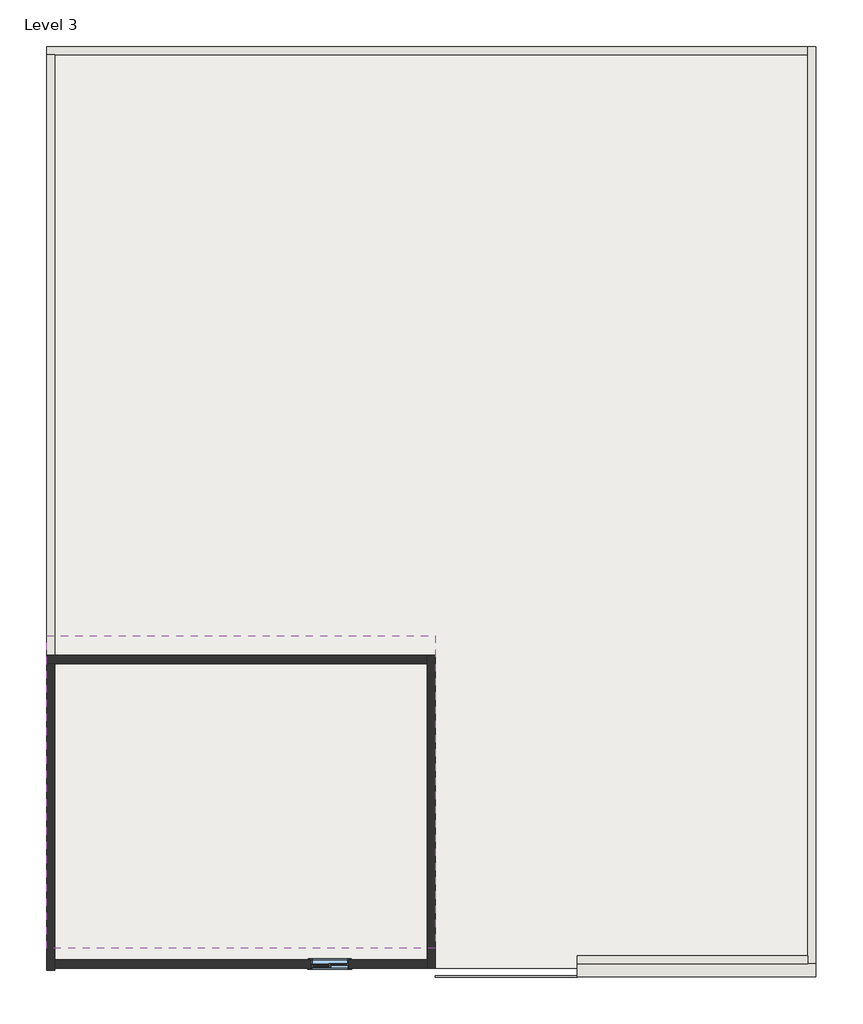
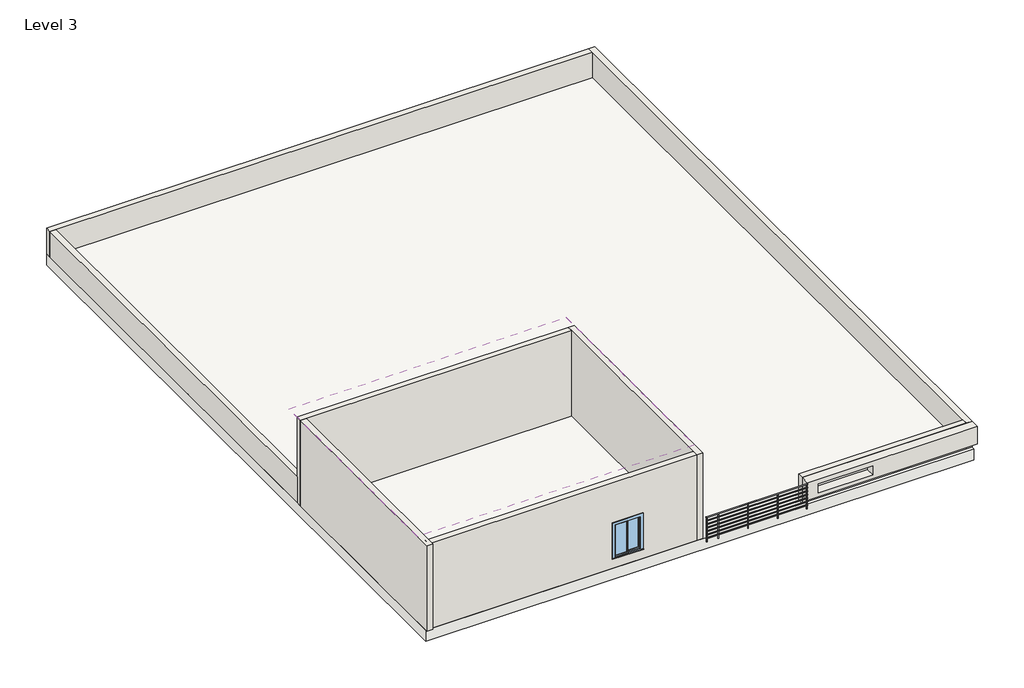
# One storey: 9 walls, 1 covering, 1 railing, 1 slab, 1 window.
"""IFC4 building model written with IfcOpenShell, lengths in millimetres."""

from ifc_helpers import new_model, si_unit, point, frame, frame_2d, origin, place, context, project, spatial, polyline, circle_curve, trimmed, segment, composite_curve, outline, extrude, faceted_brep, transform, mapped, element, save
from components import walls_8_walls_8_f603c033, window_242facca

model = new_model("IFC4")

# Units and contexts
model_context = context("Model", 3, world=origin())
ifc_project = project(units=[si_unit("LENGTHUNIT", "METRE", prefix="MILLI")], contexts=[model_context])

# Site, building, storey
site = spatial("IfcSite", under=ifc_project)
building = spatial("IfcBuilding", under=site)
storey = spatial("IfcBuildingStorey", under=building, Name="Level 3", Elevation=3048.0)

# Covering
placement = place(None, origin())
element("IfcCovering", 1, ObjectType="600 x 1200mm grid", at=placement, inside=storey, context=model_context, shape_type="SweptSolid", body=[
    extrude(outline(polyline([(-8500.3243543, 1384.0389967), (-8500.3243543, -6131.1610033), (-17844.3243543, -6131.1610033), (-17844.3243543, 1384.0389967), (-8500.3243543, 1384.0389967)])), frame((0.0, 0.0, 6096.0), z_axis=(0.0, 0.0, 1.0), x_axis=(1.0, 0.0, 0.0)), (0.0, 0.0, 1.0), 52.0),
])

# Railing
element("IfcRailing", 2, ObjectType="900mm Pipe", at=placement, inside=storey, context=model_context, shape_type="SweptSolid", body=[
    extrude(outline(composite_curve([segment(trimmed(circle_curve(frame_2d((-6810.6562913, 3928.0)), 20.0), [point((-6790.6562913, 3928.0))], [point((-6830.6562913, 3928.0))], False, "CARTESIAN"), True, "CONTINUOUS"), segment(trimmed(circle_curve(frame_2d((-6810.6562913, 3928.0)), 20.0), [point((-6830.6562913, 3928.0))], [point((-6790.6562913, 3928.0))], False, "CARTESIAN"), True, "CONTINUOUS")], self_intersect=False)), frame((-8498.4019361, 0.0, 0.0), z_axis=(1.0, 0.0, 0.0), x_axis=(0.0, 1.0, 0.0)), (0.0, 0.0, 1.0), 3405.2),
    extrude(outline(composite_curve([segment(trimmed(circle_curve(frame_2d((-6810.6562913, 3808.0)), 15.0), [point((-6825.6562913, 3808.0))], [point((-6795.6562913, 3808.0))], False, "CARTESIAN"), True, "CONTINUOUS"), segment(trimmed(circle_curve(frame_2d((-6810.6562913, 3808.0)), 15.0), [point((-6795.6562913, 3808.0))], [point((-6825.6562913, 3808.0))], False, "CARTESIAN"), True, "CONTINUOUS")], self_intersect=False)), frame((-8498.4019361, 0.0, 0.0), z_axis=(1.0, 0.0, 0.0), x_axis=(0.0, 1.0, 0.0)), (0.0, 0.0, 1.0), 3405.2),
    extrude(outline(composite_curve([segment(trimmed(circle_curve(frame_2d((-6810.6562913, 3683.0)), 15.0), [point((-6825.6562913, 3683.0))], [point((-6795.6562913, 3683.0))], False, "CARTESIAN"), True, "CONTINUOUS"), segment(trimmed(circle_curve(frame_2d((-6810.6562913, 3683.0)), 15.0), [point((-6795.6562913, 3683.0))], [point((-6825.6562913, 3683.0))], False, "CARTESIAN"), True, "CONTINUOUS")], self_intersect=False)), frame((-8498.4019361, 0.0, 0.0), z_axis=(1.0, 0.0, 0.0), x_axis=(0.0, 1.0, 0.0)), (0.0, 0.0, 1.0), 3405.2),
    extrude(outline(composite_curve([segment(trimmed(circle_curve(frame_2d((-6810.6562913, 3558.0)), 15.0), [point((-6825.6562913, 3558.0))], [point((-6795.6562913, 3558.0))], False, "CARTESIAN"), True, "CONTINUOUS"), segment(trimmed(circle_curve(frame_2d((-6810.6562913, 3558.0)), 15.0), [point((-6795.6562913, 3558.0))], [point((-6825.6562913, 3558.0))], False, "CARTESIAN"), True, "CONTINUOUS")], self_intersect=False)), frame((-8498.4019361, 0.0, 0.0), z_axis=(1.0, 0.0, 0.0), x_axis=(0.0, 1.0, 0.0)), (0.0, 0.0, 1.0), 3405.2),
    extrude(outline(composite_curve([segment(trimmed(circle_curve(frame_2d((-6810.6562913, 3433.0)), 15.0), [point((-6825.6562913, 3433.0))], [point((-6795.6562913, 3433.0))], False, "CARTESIAN"), True, "CONTINUOUS"), segment(trimmed(circle_curve(frame_2d((-6810.6562913, 3433.0)), 15.0), [point((-6795.6562913, 3433.0))], [point((-6825.6562913, 3433.0))], False, "CARTESIAN"), True, "CONTINUOUS")], self_intersect=False)), frame((-8498.4019361, 0.0, 0.0), z_axis=(1.0, 0.0, 0.0), x_axis=(0.0, 1.0, 0.0)), (0.0, 0.0, 1.0), 3405.2),
    extrude(outline(composite_curve([segment(trimmed(circle_curve(frame_2d((-6810.6562913, 3308.0)), 15.0), [point((-6825.6562913, 3308.0))], [point((-6795.6562913, 3308.0))], False, "CARTESIAN"), True, "CONTINUOUS"), segment(trimmed(circle_curve(frame_2d((-6810.6562913, 3308.0)), 15.0), [point((-6795.6562913, 3308.0))], [point((-6825.6562913, 3308.0))], False, "CARTESIAN"), True, "CONTINUOUS")], self_intersect=False)), frame((-8498.4019361, 0.0, 0.0), z_axis=(1.0, 0.0, 0.0), x_axis=(0.0, 1.0, 0.0)), (0.0, 0.0, 1.0), 3405.2),
    extrude(outline(composite_curve([segment(trimmed(circle_curve(frame_2d((-6810.6562913, 3183.0)), 15.0), [point((-6825.6562913, 3183.0))], [point((-6795.6562913, 3183.0))], False, "CARTESIAN"), True, "CONTINUOUS"), segment(trimmed(circle_curve(frame_2d((-6810.6562913, 3183.0)), 15.0), [point((-6795.6562913, 3183.0))], [point((-6825.6562913, 3183.0))], False, "CARTESIAN"), True, "CONTINUOUS")], self_intersect=False)), frame((-8498.4019361, 0.0, 0.0), z_axis=(1.0, 0.0, 0.0), x_axis=(0.0, 1.0, 0.0)), (0.0, 0.0, 1.0), 3405.2),
    extrude(outline(composite_curve([segment(trimmed(circle_curve(frame_2d((-8093.2019361, -6810.6562913)), 12.5), [point((-8093.2019361, -6823.1562913))], [point((-8093.2019361, -6798.1562913))], False, "CARTESIAN"), True, "CONTINUOUS"), segment(trimmed(circle_curve(frame_2d((-8093.2019361, -6810.6562913)), 12.5), [point((-8093.2019361, -6798.1562913))], [point((-8093.2019361, -6823.1562913))], False, "CARTESIAN"), True, "CONTINUOUS")], self_intersect=False)), frame((0.0, 0.0, 3048.0), z_axis=(0.0, 0.0, 1.0), x_axis=(1.0, 0.0, 0.0)), (0.0, 0.0, 1.0), 860.0),
    extrude(outline(composite_curve([segment(trimmed(circle_curve(frame_2d((-7093.2019361, -6810.6562913)), 12.5), [point((-7093.2019361, -6823.1562913))], [point((-7093.2019361, -6798.1562913))], False, "CARTESIAN"), True, "CONTINUOUS"), segment(trimmed(circle_curve(frame_2d((-7093.2019361, -6810.6562913)), 12.5), [point((-7093.2019361, -6798.1562913))], [point((-7093.2019361, -6823.1562913))], False, "CARTESIAN"), True, "CONTINUOUS")], self_intersect=False)), frame((0.0, 0.0, 3048.0), z_axis=(0.0, 0.0, 1.0), x_axis=(1.0, 0.0, 0.0)), (0.0, 0.0, 1.0), 860.0),
    extrude(outline(composite_curve([segment(trimmed(circle_curve(frame_2d((-6093.2019361, -6810.6562913)), 12.5), [point((-6093.2019361, -6823.1562913))], [point((-6093.2019361, -6798.1562913))], False, "CARTESIAN"), True, "CONTINUOUS"), segment(trimmed(circle_curve(frame_2d((-6093.2019361, -6810.6562913)), 12.5), [point((-6093.2019361, -6798.1562913))], [point((-6093.2019361, -6823.1562913))], False, "CARTESIAN"), True, "CONTINUOUS")], self_intersect=False)), frame((0.0, 0.0, 3048.0), z_axis=(0.0, 0.0, 1.0), x_axis=(1.0, 0.0, 0.0)), (0.0, 0.0, 1.0), 860.0),
    extrude(outline(composite_curve([segment(trimmed(circle_curve(frame_2d((-8485.9019361, -6810.6562913)), 12.5), [point((-8485.9019361, -6823.1562913))], [point((-8485.9019361, -6798.1562913))], False, "CARTESIAN"), True, "CONTINUOUS"), segment(trimmed(circle_curve(frame_2d((-8485.9019361, -6810.6562913)), 12.5), [point((-8485.9019361, -6798.1562913))], [point((-8485.9019361, -6823.1562913))], False, "CARTESIAN"), True, "CONTINUOUS")], self_intersect=False)), frame((0.0, 0.0, 3048.0), z_axis=(0.0, 0.0, 1.0), x_axis=(1.0, 0.0, 0.0)), (0.0, 0.0, 1.0), 860.0),
    extrude(outline(composite_curve([segment(trimmed(circle_curve(frame_2d((-5105.7019361, -6810.6562913)), 12.5), [point((-5105.7019361, -6823.1562913))], [point((-5105.7019361, -6798.1562913))], False, "CARTESIAN"), True, "CONTINUOUS"), segment(trimmed(circle_curve(frame_2d((-5105.7019361, -6810.6562913)), 12.5), [point((-5105.7019361, -6798.1562913))], [point((-5105.7019361, -6823.1562913))], False, "CARTESIAN"), True, "CONTINUOUS")], self_intersect=False)), frame((0.0, 0.0, 3048.0), z_axis=(0.0, 0.0, 1.0), x_axis=(1.0, 0.0, 0.0)), (0.0, 0.0, 1.0), 860.0),
])

# Slab
element("IfcSlab", 3, ObjectType="Generic Floor - 400mm", at=placement, inside=storey, context=model_context, shape_type="SweptSolid", body=[
    extrude(outline(polyline([(645.5980639, 15539.7437087), (645.5980639, -6605.8562913), (-17842.4019361, -6605.8562913), (-17842.4019361, 15539.7437087), (645.5980639, 15539.7437087)])), frame((0.0, 0.0, 2648.0), z_axis=(0.0, 0.0, 1.0), x_axis=(1.0, 0.0, 0.0)), (0.0, 0.0, 1.0), 400.0),
])

# Walls
element("IfcWall", 4, ObjectType="Generic - 200mm", at=placement, inside=storey, context=model_context, shape_type="Brep", body=[
    faceted_brep([(-17842.4019361, 15339.7437087, 3048.0), (-17642.4019361, 15339.7437087, 3048.0), (445.5980639, 15339.7437087, 3048.0), (445.5980639, 15339.7437087, 3962.4), (-17642.4019361, 15339.7437087, 3962.4), (-17842.4019361, 15339.7437087, 3962.4), (-17842.4019361, 15539.7437087, 3048.0), (-17842.4019361, 15539.7437087, 3962.4), (445.5980639, 15539.7437087, 3962.4), (445.5980639, 15539.7437087, 3048.0)], [[[0, 1, 2, 3, 4, 5]], [[6, 7, 8, 9]], [[2, 1, 0, 6, 9]], [[5, 4, 3, 8, 7]], [[0, 5, 7, 6]], [[3, 2, 9, 8]]]),
])
element("IfcWall", 5, ObjectType="Generic - 200mm", at=placement, inside=storey, context=model_context, shape_type="SweptSolid", body=[
    extrude(outline(polyline([(-17642.4019361, 15339.7437087), (-17642.4019361, 909.3437087), (-17842.4019361, 909.3437087), (-17842.4019361, 15339.7437087), (-17642.4019361, 15339.7437087)])), frame((0.0, 0.0, 3048.0), z_axis=(0.0, 0.0, 1.0), x_axis=(1.0, 0.0, 0.0)), (0.0, 0.0, 1.0), 914.4),
])
element("IfcWall", 6, ObjectType="Generic - 200mm", at=placement, inside=storey, context=model_context, shape_type="SweptSolid", body=[
    extrude(outline(polyline([(3048.0, -8698.4019361), (6096.0, -8698.4019361), (6096.0, -17742.4019361), (3048.0, -17742.4019361), (3048.0, -8698.4019361)]), holes=[polyline([(4609.6105054, -11494.0019361), (4609.6105054, -10579.6019361), (3390.4105054, -10579.6019361), (3390.4105054, -11494.0019361), (4609.6105054, -11494.0019361)])]), frame((0.0, -6605.8562913, 0.0), z_axis=(0.0, 1.0, 0.0), x_axis=(0.0, 0.0, 1.0)), (0.0, 0.0, 1.0), 200.0),
])
element("IfcWall", 7, ObjectType="Generic - 200mm", at=placement, inside=storey, context=model_context, shape_type="Brep", body=[
    faceted_brep([(445.5980639, 15539.7437087, 3048.0), (445.5980639, 15339.7437087, 3048.0), (445.5980639, -6305.8562913, 3048.0), (445.5980639, -6505.8562913, 3048.0), (445.5980639, -6505.8562913, 3969.8902454), (445.5980639, -6305.8562913, 3969.8902454), (445.5980639, 15539.7437087, 3969.8902454), (445.5980639, 15539.7437087, 3962.4), (645.5980639, 15539.7437087, 3048.0), (645.5980639, 15539.7437087, 3969.8902454), (645.5980639, -6505.8562913, 3969.8902454), (645.5980639, -6505.8562913, 3048.0)], [[[0, 1, 2, 3, 4, 5, 6, 7]], [[8, 9, 10, 11]], [[3, 2, 1, 0, 8, 11]], [[6, 5, 4, 10, 9]], [[0, 7, 6, 9, 8]], [[4, 3, 11, 10]]]),
])
element("IfcWall", 8, ObjectType="Generic - 200mm", at=placement, inside=storey, context=model_context, shape_type="Brep", body=[
    faceted_brep([(-8498.4019361, -6605.8562913, 3048.0), (-8498.4019361, 909.3437087, 3048.0), (-8498.4019361, 909.3437087, 6096.0), (-8498.4019361, -6605.8562913, 6096.0), (-8698.4019361, -6605.8562913, 3048.0), (-8698.4019361, -6605.8562913, 6096.0), (-8698.4019361, -6405.8562913, 6096.0), (-8698.4019361, 709.3437087, 6096.0), (-8698.4019361, 909.3437087, 6096.0), (-8698.4019361, 909.3437087, 3048.0), (-8698.4019361, 709.3437087, 3048.0), (-8698.4019361, -6405.8562913, 3048.0)], [[[0, 1, 2, 3]], [[4, 5, 6, 7, 8, 9, 10, 11]], [[1, 0, 4, 11, 10, 9]], [[3, 2, 8, 7, 6, 5]], [[0, 3, 5, 4]], [[2, 1, 9, 8]]]),
])
element("IfcWall", 9, ObjectType="Generic - 200mm", at=placement, inside=storey, context=model_context, shape_type="Brep", body=[
    faceted_brep([(-8698.4019361, 909.3437087, 3048.0), (-17642.4019361, 909.3437087, 3048.0), (-17842.4019361, 909.3437087, 3048.0), (-17842.4019361, 909.3437087, 3962.4), (-17842.4019361, 909.3437087, 6096.0), (-8698.4019361, 909.3437087, 6096.0), (-8698.4019361, 709.3437087, 3048.0), (-8698.4019361, 709.3437087, 6096.0), (-17642.4019361, 709.3437087, 6096.0), (-17842.4019361, 709.3437087, 6096.0), (-17842.4019361, 709.3437087, 3048.0), (-17642.4019361, 709.3437087, 3048.0)], [[[0, 1, 2, 3, 4, 5]], [[6, 7, 8, 9, 10, 11]], [[2, 1, 0, 6, 11, 10]], [[5, 4, 9, 8, 7]], [[0, 5, 7, 6]], [[2, 10, 9, 4, 3]]]),
])
element("IfcWall", 10, ObjectType="Generic - 200mm", at=placement, inside=storey, context=model_context, shape_type="SweptSolid", body=[
    extrude(outline(polyline([(-5093.2019361, -6305.8562913), (445.5980639, -6305.8562913), (445.5980639, -6505.8562913), (-5093.2019361, -6505.8562913), (-5093.2019361, -6305.8562913)])), frame((0.0, 0.0, 3048.0), z_axis=(0.0, 0.0, 1.0), x_axis=(1.0, 0.0, 0.0)), (0.0, 0.0, 1.0), 921.8902454),
])
element("IfcWall", 11, ObjectType="Generic - 200mm", at=placement, inside=storey, context=model_context, shape_type="SweptSolid", body=[
    extrude(outline(polyline([(-17842.4019361, -6658.2562913), (-17842.4019361, 709.3437087), (-17642.4019361, 709.3437087), (-17642.4019361, -6658.2562913), (-17842.4019361, -6658.2562913)])), frame((0.0, 0.0, 3048.0), z_axis=(0.0, 0.0, 1.0), x_axis=(1.0, 0.0, 0.0)), (0.0, 0.0, 1.0), 3048.0),
])
walls_8_walls_8_shape = walls_8_walls_8_f603c033(model_context)
element("IfcWall", 12, ObjectType="Walls 8 : Walls 8", at=placement, inside=storey, context=model_context, shape_type="MappedRepresentation", body=[
    mapped(walls_8_walls_8_shape, transform((0.0, 0.0, 0.0), x_axis=(1.0, 0.0, 0.0), y_axis=(0.0, 1.0, 0.0), z_axis=(0.0, 0.0, 1.0))),
])

# Window
window_shape = window_242facca(model_context)
element("IfcWindow", 13, ObjectType="Slider with Trim : 36\" x 48\"", at=placement, inside=storey, context=model_context, shape_type="MappedRepresentation", body=[
    mapped(window_shape, transform((-11036.8019361, -6505.8562913, 2476.0105054), x_axis=(-1.0, 0.0, 0.0), y_axis=(0.0, -1.0, 0.0), z_axis=(0.0, 0.0, 1.0))),
])

save(model, "model.ifc")

# Revit data of these elements
# Type "600 x 1200mm grid"
#   built-in parameter 1002203 = 1 (stored number, unit not read)
#   built-in parameter 1002202 = 1 (stored number, unit not read)
#   Layers, outside or top first: 0' - 1.41732" "Default" (function 1); 0' - 0.62992" "Ceiling Tile 600 x 1200" (function 5)
# Type "900mm Pipe"
#   built-in parameter 1008612 = 0.019685 (stored number, unit not read)
#   built-in parameter 1008611 = 0.0984252 (stored number, unit not read)
#   built-in parameter 1008609 = 6.56168 (stored number, unit not read)
#   built-in parameter 1008604 = 0.19685 (stored number, unit not read)
#   built-in parameter 1008603 = 0.164042 (stored number, unit not read)
#   Railing Height = 2' - 11.43307"
#   built-in parameter 1008630 = 2
#   built-in parameter 1008610 = 2
#   built-in parameter 1008605 = 1
#   built-in parameter 1008618 = M_Baluster - Round : 25mm
# Type "Generic Floor - 400mm"
#   Function = 0
#   Layers, outside or top first: 1' - 3.74803" no material (function 1)
# Type "Generic - 200mm"
#   Layers, outside or top first: 0' - 7.87402" no material (function 1)
# Type "Slider with Trim : 36\" x 48\""
#   Type Mark = "19"
#   Construction Type Id = "GSP4R"
#   Assembly Code = "B2020100"
#   Analytic Construction = "1/8 in Pilkington single glazing"
#   Visual Light Transmittance = 0.9
#   Solar Heat Gain Coefficient = 0.78
#   Heat Transfer Coefficient (U) = 3.6886 W/(m²·K)
#   Height = 4' - 0"
#   Default Sill Height = 3' - 0"
#   Trim Projection - Ext. = 0' - 0 3/4"
#   Trim Projection - Int. = 0' - 0 3/4"
#   Trim Width - Exterior = 0' - 3 1/2"
#   Trim Width - Interior = 0' - 3 1/2"
#   Width = 3' - 0"
#   Window Inset = 0' - 0 3/4"
#   Define Thermal Properties by = 1
#   Glass Pane Material = Glass
#   Sash Material = Sash
#   Trim Exterior Material = Trim
#   Trim Interior Material = Trim
#   Wall Closure = (empty or 0)
# Element 1 (IfcCovering, "600 x 1200mm grid")
#   Height Offset From Level = 10' - 0"
#   Phase Created = New Construction
#   Materials on its faces: "Ceiling Tile 600 x 1200", "Default"
# Element 2 (IfcRailing, "900mm Pipe")
#   Phase Created = New Construction
# Element 3 (IfcSlab, "Generic Floor - 400mm")
#   Height Offset From Level = 0' - 0"
#   Phase Created = New Construction
#   Materials on its faces: "Default Roof"
# Elements 4, 5 (IfcWall, "Generic - 200mm")
#   Top Offset = 0' - 0"
#   Base Offset = 0' - 0"
#   Unconnected Height = 3' - 0"
#   wall height = 3' - 0"
#   Phase Created = New Construction
#   Base Constraint = Level 3
#   Materials on its faces: "Default Wall"
# Elements 6, 8, 9, 11 (IfcWall, "Generic - 200mm")
#   Top Offset = 0' - 0"
#   Base Offset = 0' - 0"
#   Unconnected Height = 10' - 0"
#   wall height = 10' - 0"
#   Phase Created = New Construction
#   Base Constraint = Level 3
#   Materials on its faces: "Default Wall"
# Elements 7, 10 (IfcWall, "Generic - 200mm")
#   Top Offset = 0' - 0"
#   Base Offset = 0' - 0"
#   Unconnected Height = 3' - 0.29489"
#   wall height = 3' - 0.29489"
#   Phase Created = New Construction
#   Base Constraint = Level 3
#   Materials on its faces: "Default Wall"
# Element 12 (IfcWall, "Walls 8 : Walls 8")
#   Phase Created = New Construction
#   Materials on its faces: "Default Wall"
# Element 13 (IfcWindow, "Slider with Trim : 36\" x 48\"")
#   Mark = "6"
#   Phase Created = New Construction
#   Materials on its faces: "Sash", "Trim", "Glass"
# Materials
#   "Default": colour RGB 80 80 80, transparency 0
#   "Ceiling Tile 600 x 1200": class "Generic", colour RGB 179 178 175, transparency 0, Description = "Acoustic ceiling tile", Cost = 0
#   "Glass": class "Glass", colour RGB 218 227 224, transparency 0.85, Description = "Soda Lime Glass", Cost = 0
#   "Sash": class "Wood", colour RGB 136 99 55, transparency 0
#   "Trim": class "Wood", colour RGB 224 178 126, transparency 0
#   "Default Roof": colour RGB 80 80 80, transparency 0
#   "Default Wall": colour RGB 80 80 80, transparency 0
